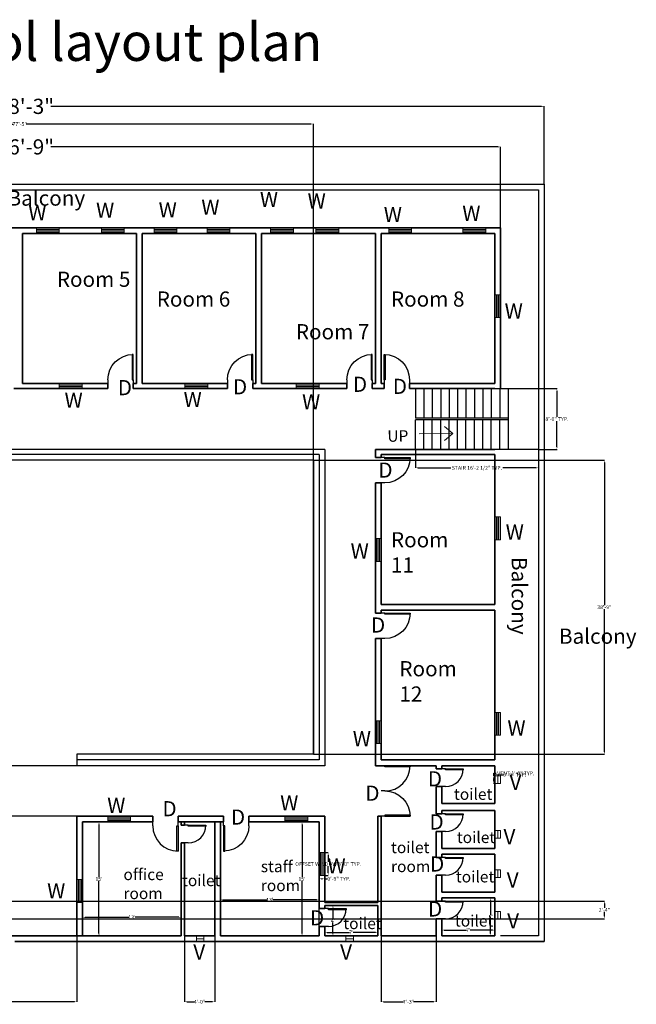
# Model space of a CAD drawing. Units: inches. Extents: x 6562 to 8578, y 2662 to 4218.
# Tile 3 of 3: x 7603 to 8578, y 2662 to 4218. Entities that reach past the tile are written whole.
import ezdxf

# ---------------------------------------------------------------- set-up
doc = ezdxf.new("R2010")
doc.units = ezdxf.units.IN
doc.header["$MEASUREMENT"] = 0
for name, color, linetype, lineweight in [('A-ANNO-DIMS', 2, 'Continuous', 18), ('A-ANNO-SYMB', 2, 'Continuous', 18), ('A-ANNO-TEXT', 7, 'Continuous', 18), ('A-AREA-IDEN', 7, 'Continuous', 25), ('A-DOOR', 3, 'Continuous', 25), ('A-FLOR-EDGE', 8, 'Continuous', 25), ('A-FLOR-STRS', 7, 'Continuous', 25), ('A-GLAZ', 4, 'Continuous', 18), ('A-GLAZ-VENT', 4, 'Continuous', 18), ('A-WALL', 7, 'Continuous', 35)]:
    doc.layers.add(name, color=color, linetype=linetype, lineweight=lineweight)
doc.styles.get("Standard").update_dxf_attribs({"font": 'arial.ttf'})
doc.dimstyles.get("Standard").update_dxf_attribs({"dimtxt": 6, "dimasz": 4, "dimexe": 0.18, "dimexo": 0.0625, "dimgap": 0.09, "dimtad": 0, "dimtih": 1, "dimtoh": 1, "dimdec": 0, "dimzin": 0, "dimdsep": 46, "dimlunit": 3, "dimtxsty": 'Standard', "dimcen": 0.09, "dimadec": 0, "dimazin": 0, "dimtfac": 1, "dimtdec": 0, "dimtofl": 0, "dimtmove": 0, "dimatfit": 3, "dimfxl": 1, "dimtolj": 1, "dimtzin": 0, "dimarcsym": 0})

# ---------------------------------------------------------------- blocks, each defined once
blk = doc.blocks.new('*U4')
for p, q in [((-40, 0), (-40, 6)), ((0, 0), (0, 6))]:
    blk.add_line(p, q)
blk.add_lwpolyline([(0, 0), (0, -40), (-1.75, -40), (-1.75, 0)], close=True)
blk.add_arc((0, 0), 40, 180, 270)
blk = doc.blocks.new('*U5')
for p, q in [((-28, 0), (-28, 6)), ((0, 0), (0, 6))]:
    blk.add_line(p, q)
blk.add_lwpolyline([(0, 0), (0, -28), (-1.75, -28), (-1.75, 0)], close=True)
blk.add_arc((0, 0), 28, 180, 270)
blk = doc.blocks.new('*U2')
for p, q in [((0, 0), (0, -6)), ((40, 0), (40, -6))]:
    blk.add_line(p, q)
blk.add_lwpolyline([(0, 0), (0, 40), (1.75, 40), (1.75, 0)], close=True)
blk.add_arc((0, 0), 40, 0, 90)
blk = doc.blocks.new('*U6')
for p, q in [((0, 0), (0, -6)), ((28, 0), (28, -6))]:
    blk.add_line(p, q)
blk.add_lwpolyline([(0, 0), (0, 28), (1.75, 28), (1.75, 0)], close=True)
blk.add_arc((0, 0), 28, 0, 90)
blk = doc.blocks.new('*U8')
for p, q in [((0, 0), (0, -6)), ((40, 0), (40, -6))]:
    blk.add_line(p, q)
blk.add_lwpolyline([(0, 0), (0, 40), (1.75, 40), (1.75, 0)], close=True)
blk.add_arc((0, 0), 40, 0, 90)
blk = doc.blocks.new('*U9')
for p, q in [((0, 0), (0, -6)), ((-40, 0), (-40, -6))]:
    blk.add_line(p, q)
blk.add_lwpolyline([(0, 0), (0, 40), (-1.75, 40), (-1.75, 0)], close=True)
blk.add_arc((0, 0), 40, 90, 180)
blk = doc.blocks.new('*U10')
for p, q in [((0, 0), (0, 6)), ((40, 0), (40, 6))]:
    blk.add_line(p, q)
blk.add_lwpolyline([(0, 0), (0, -40), (1.75, -40), (1.75, 0)], close=True)
blk.add_arc((0, 0), 40, 270, 0)
blk = doc.blocks.new('*D11')
at = {"layer": 'A-ANNO-DIMS', "color": 0, "lineweight": -2, "transparency": 16777216}
for p, q in [((6773.2, 3958.1), (6773.2, 4081.4)), ((6777.2, 4081.2), (7553.2, 4081.2)), ((8428.2, 4081.2), (7652.2, 4081.2)), ((8432.2, 3958.1), (8432.2, 4081.4))]:
    blk.add_line(p, q, dxfattribs=at)
at = {"layer": 'A-ANNO-DIMS', "color": 0, "transparency": 16777216}
for points in [[(6777.2, 4081.9), (6777.2, 4080.6), (6773.2, 4081.2)], [(8428.2, 4081.9), (8428.2, 4080.6), (8432.2, 4081.2)]]:
    blk.add_solid(points, dxfattribs=at)
at = {"layer": 'Defpoints', "color": 0, "transparency": 16777216}
for p in [(8432.2, 4081.2), (6773.2, 3958), (8432.2, 3958)]:
    blk.add_point(p, dxfattribs=at)
at = {"layer": 'A-ANNO-DIMS', "color": 0, "transparency": 16777216, "insert": (7602.7, 4081.2), "char_height": 6, "attachment_point": 5}
blk.add_mtext('\\A1;{\\H4x;138\'-3"}', dxfattribs=at)
blk = doc.blocks.new('*D12')
at = {"layer": 'A-ANNO-DIMS', "color": 0, "lineweight": -2, "transparency": 16777216}
for p, q in [((6842.2, 3889.1), (6842.2, 4017.3)), ((6846.2, 4017.1), (7553.2, 4017.1)), ((8359.2, 4017.1), (7652.2, 4017.1)), ((8363.2, 3889.1), (8363.2, 4017.3))]:
    blk.add_line(p, q, dxfattribs=at)
at = {"layer": 'A-ANNO-DIMS', "color": 0, "transparency": 16777216}
for points in [[(6846.2, 4017.8), (6846.2, 4016.4), (6842.2, 4017.1)], [(8359.2, 4017.8), (8359.2, 4016.4), (8363.2, 4017.1)]]:
    blk.add_solid(points, dxfattribs=at)
at = {"layer": 'Defpoints', "color": 0, "transparency": 16777216}
for p in [(8363.2, 4017.1), (6842.2, 3889), (8363.2, 3889)]:
    blk.add_point(p, dxfattribs=at)
at = {"layer": 'A-ANNO-DIMS', "color": 0, "transparency": 16777216, "insert": (7602.7, 4017.1), "char_height": 6, "attachment_point": 5}
blk.add_mtext('\\A1;{\\H4x;126\'-9"}', dxfattribs=at)
blk = doc.blocks.new('*D17')
at = {"layer": 'A-ANNO-DIMS', "color": 0, "lineweight": -2, "transparency": 16777216}
for p, q in [((7702.2, 2770.1), (7702.2, 2799.6)), ((7706.2, 2799.4), (7775.3, 2799.4)), ((7854.2, 2799.4), (7785.1, 2799.4)), ((7858.2, 2770.1), (7858.2, 2799.6))]:
    blk.add_line(p, q, dxfattribs=at)
at = {"layer": 'A-ANNO-DIMS', "color": 0, "transparency": 16777216}
for points in [[(7706.2, 2800.1), (7706.2, 2798.8), (7702.2, 2799.4)], [(7854.2, 2800.1), (7854.2, 2798.8), (7858.2, 2799.4)]]:
    blk.add_solid(points, dxfattribs=at)
at = {"layer": 'Defpoints', "color": 0, "transparency": 16777216}
for p in [(7858.2, 2799.4), (7702.2, 2770), (7858.2, 2770)]:
    blk.add_point(p, dxfattribs=at)
at = {"layer": 'A-ANNO-DIMS', "color": 0, "transparency": 16777216, "insert": (7780.2, 2799.4), "char_height": 6, "attachment_point": 5}
blk.add_mtext("\\A1;13'", dxfattribs=at)
blk = doc.blocks.new('*D18')
at = {"layer": 'A-ANNO-DIMS', "color": 0, "lineweight": -2, "transparency": 16777216}
for p, q in [((7702.2, 2950), (7728.3, 2950)), ((7728.1, 2946), (7728.1, 2863.2)), ((7728.1, 2774), (7728.1, 2856.8)), ((7702.2, 2770), (7728.3, 2770))]:
    blk.add_line(p, q, dxfattribs=at)
at = {"layer": 'A-ANNO-DIMS', "color": 0, "transparency": 16777216}
for points in [[(7727.5, 2946), (7728.8, 2946), (7728.1, 2950)], [(7727.5, 2774), (7728.8, 2774), (7728.1, 2770)]]:
    blk.add_solid(points, dxfattribs=at)
at = {"layer": 'Defpoints', "color": 0, "transparency": 16777216}
for p in [(7702.2, 2950), (7702.2, 2770), (7728.1, 2770)]:
    blk.add_point(p, dxfattribs=at)
at = {"layer": 'A-ANNO-DIMS', "color": 0, "transparency": 16777216, "insert": (7728.1, 2860), "char_height": 6, "attachment_point": 5}
blk.add_mtext("\\A1;15'", dxfattribs=at)
blk = doc.blocks.new('*D21')
at = {"layer": 'A-ANNO-DIMS', "color": 0, "lineweight": -2, "transparency": 16777216}
for p, q in [((7920.2, 2770.1), (7920.2, 2827.1)), ((7924.2, 2826.9), (7993.3, 2826.9)), ((8072.2, 2826.9), (8003.1, 2826.9)), ((8076.2, 2770.1), (8076.2, 2827.1))]:
    blk.add_line(p, q, dxfattribs=at)
at = {"layer": 'A-ANNO-DIMS', "color": 0, "transparency": 16777216}
for points in [[(7924.2, 2827.6), (7924.2, 2826.2), (7920.2, 2826.9)], [(8072.2, 2827.6), (8072.2, 2826.2), (8076.2, 2826.9)]]:
    blk.add_solid(points, dxfattribs=at)
at = {"layer": 'Defpoints', "color": 0, "transparency": 16777216}
for p in [(8076.2, 2826.9), (7920.2, 2770), (8076.2, 2770)]:
    blk.add_point(p, dxfattribs=at)
at = {"layer": 'A-ANNO-DIMS', "color": 0, "transparency": 16777216, "insert": (7998.2, 2826.9), "char_height": 6, "attachment_point": 5}
blk.add_mtext("\\A1;13'", dxfattribs=at)
blk = doc.blocks.new('*D22')
at = {"layer": 'A-ANNO-DIMS', "color": 0, "lineweight": -2, "transparency": 16777216}
for p, q in [((8076.1, 2950), (8049.1, 2950)), ((8049.2, 2946), (8049.2, 2863.2)), ((8049.2, 2774), (8049.2, 2856.8)), ((8076.1, 2770), (8049.1, 2770))]:
    blk.add_line(p, q, dxfattribs=at)
at = {"layer": 'A-ANNO-DIMS', "color": 0, "transparency": 16777216}
for points in [[(8048.6, 2946), (8049.9, 2946), (8049.2, 2950)], [(8048.6, 2774), (8049.9, 2774), (8049.2, 2770)]]:
    blk.add_solid(points, dxfattribs=at)
at = {"layer": 'Defpoints', "color": 0, "transparency": 16777216}
for p in [(8076.2, 2950), (8049.2, 2770), (8076.2, 2770)]:
    blk.add_point(p, dxfattribs=at)
at = {"layer": 'A-ANNO-DIMS', "color": 0, "transparency": 16777216, "insert": (8049.2, 2860), "char_height": 6, "attachment_point": 5}
blk.add_mtext("\\A1;15'", dxfattribs=at)
blk = doc.blocks.new('*D23')
at = {"layer": 'A-ANNO-DIMS', "color": 0, "lineweight": -2, "transparency": 16777216}
for p, q in [((8169.1, 2818), (8098, 2818)), ((8098.2, 2814), (8098.2, 2797.1)), ((8098.2, 2774), (8098.2, 2790.9)), ((8169.1, 2770), (8098, 2770))]:
    blk.add_line(p, q, dxfattribs=at)
at = {"layer": 'A-ANNO-DIMS', "color": 0, "transparency": 16777216}
for points in [[(8097.5, 2814), (8098.8, 2814), (8098.2, 2818)], [(8097.5, 2774), (8098.8, 2774), (8098.2, 2770)]]:
    blk.add_solid(points, dxfattribs=at)
at = {"layer": 'Defpoints', "color": 0, "transparency": 16777216}
for p in [(8169.2, 2818), (8098.2, 2770), (8169.2, 2770)]:
    blk.add_point(p, dxfattribs=at)
at = {"layer": 'A-ANNO-DIMS', "color": 0, "transparency": 16777216, "insert": (8098.2, 2794), "char_height": 6, "attachment_point": 5}
blk.add_mtext("\\A1;4'", dxfattribs=at)
blk = doc.blocks.new('*D24')
at = {"layer": 'A-ANNO-DIMS', "color": 0, "lineweight": -2, "transparency": 16777216}
for p, q in [((8085.2, 2770.1), (8085.2, 2775.7)), ((8089.2, 2775.5), (8124.4, 2775.5)), ((8165.2, 2775.5), (8130, 2775.5)), ((8169.2, 2770.1), (8169.2, 2775.7))]:
    blk.add_line(p, q, dxfattribs=at)
at = {"layer": 'A-ANNO-DIMS', "color": 0, "transparency": 16777216}
for points in [[(8089.2, 2776.1), (8089.2, 2774.8), (8085.2, 2775.5)], [(8165.2, 2776.1), (8165.2, 2774.8), (8169.2, 2775.5)]]:
    blk.add_solid(points, dxfattribs=at)
at = {"layer": 'Defpoints', "color": 0, "transparency": 16777216}
for p in [(8169.2, 2775.5), (8085.2, 2770), (8169.2, 2770)]:
    blk.add_point(p, dxfattribs=at)
at = {"layer": 'A-ANNO-DIMS', "color": 0, "transparency": 16777216, "insert": (8127.2, 2775.5), "char_height": 6, "attachment_point": 5}
blk.add_mtext("\\A1;7'", dxfattribs=at)
blk = doc.blocks.new('*D25')
at = {"layer": 'A-ANNO-DIMS', "color": 0, "lineweight": -2, "transparency": 16777216}
for p, q in [((8270.2, 2770.1), (8270.2, 2779.3)), ((8274.2, 2779.1), (8309.4, 2779.1)), ((8350.2, 2779.1), (8315, 2779.1)), ((8354.2, 2770.1), (8354.2, 2779.3))]:
    blk.add_line(p, q, dxfattribs=at)
at = {"layer": 'A-ANNO-DIMS', "color": 0, "transparency": 16777216}
for points in [[(8274.2, 2779.8), (8274.2, 2778.4), (8270.2, 2779.1)], [(8350.2, 2779.8), (8350.2, 2778.4), (8354.2, 2779.1)]]:
    blk.add_solid(points, dxfattribs=at)
at = {"layer": 'Defpoints', "color": 0, "transparency": 16777216}
for p in [(8354.2, 2779.1), (8270.2, 2770), (8354.2, 2770)]:
    blk.add_point(p, dxfattribs=at)
at = {"layer": 'A-ANNO-DIMS', "color": 0, "transparency": 16777216, "insert": (8312.2, 2779.1), "char_height": 6, "attachment_point": 5}
blk.add_mtext("\\A1;7'", dxfattribs=at)
blk = doc.blocks.new('*D26')
at = {"layer": 'A-ANNO-DIMS', "color": 0, "lineweight": -2, "transparency": 16777216}
for p, q in [((8354.1, 2830), (8347.2, 2830)), ((8347.4, 2826), (8347.4, 2803.1)), ((8347.4, 2774), (8347.4, 2796.9)), ((8354.1, 2770), (8347.2, 2770))]:
    blk.add_line(p, q, dxfattribs=at)
at = {"layer": 'A-ANNO-DIMS', "color": 0, "transparency": 16777216}
for points in [[(8346.7, 2826), (8348, 2826), (8347.4, 2830)], [(8346.7, 2774), (8348, 2774), (8347.4, 2770)]]:
    blk.add_solid(points, dxfattribs=at)
at = {"layer": 'Defpoints', "color": 0, "transparency": 16777216}
for p in [(8354.2, 2830), (8347.4, 2770), (8354.2, 2770)]:
    blk.add_point(p, dxfattribs=at)
at = {"layer": 'A-ANNO-DIMS', "color": 0, "transparency": 16777216, "insert": (8347.4, 2800), "char_height": 6, "attachment_point": 5}
blk.add_mtext("\\A1;5'", dxfattribs=at)
blk = doc.blocks.new('WIN-36-FRAMED')
for p, q in [((2.5, 36), (2.5, 0)), ((4.5, 36), (4.5, 0)), ((6.5, 36), (6.5, 0))]:
    blk.add_line(p, q)
blk.add_lwpolyline([(0, 36), (9, 36), (9, 0), (0, 0)], close=True)
blk = doc.blocks.new('STAIR-HALF-TURN')
for p, q in [((0, 96), (194.7, 96)), ((0, 96), (0, 49.3)), ((13.3, 96), (13.3, 49.3)), ((26.7, 96), (26.7, 49.3)), ((40, 96), (40, 49.3)), ((53.3, 96), (53.3, 49.3)), ((66.7, 96), (66.7, 49.3)), ((80, 96), (80, 49.3)), ((93.3, 96), (93.3, 49.3)), ((106.7, 96), (106.7, 49.3)), ((120, 96), (120, 49.3)), ((133.3, 96), (133.3, 49.3)), ((146.7, 96), (146.7, 48)), ((194.7, 96), (194.7, 48)), ((146.7, 49.3), (0, 49.3)), ((146.7, 48), (146.7, 0)), ((194.7, 48), (194.7, 0)), ((0, 0), (0, 46.7)), ((146.7, 46.7), (0, 46.7)), ((13.3, 0), (13.3, 46.7)), ((26.7, 0), (26.7, 46.7)), ((40, 0), (40, 46.7)), ((53.3, 0), (53.3, 46.7)), ((66.7, 0), (66.7, 46.7)), ((80, 0), (80, 46.7)), ((93.3, 0), (93.3, 46.7)), ((106.7, 0), (106.7, 46.7)), ((120, 0), (120, 46.7)), ((133.3, 0), (133.3, 46.7)), ((194.7, 0), (0, 0))]:
    blk.add_line(p, q)
blk = doc.blocks.new('VENT-12')
blk.add_line((4.5, 12), (4.5, 0))
blk.add_lwpolyline([(0, 12), (9, 12), (9, 0), (0, 0)], close=True)
blk = doc.blocks.new('WIN-36-VERANDA')
for p, q in [((0, 0), (0, 7.9)), ((36, 5.5), (0, 5.5)), ((36, 3.5), (0, 3.5)), ((36, 1.5), (0, 1.5)), ((36, 8), (36, 0))]:
    blk.add_line(p, q)
blk = doc.blocks.new('ARROW-STAIR-UP')
for p, q in [((0, 11.1), (13.3, 22.2)), ((53.3, 11.1), (0, 11.1)), ((0, 11.1), (13.3, 0))]:
    blk.add_line(p, q)
blk = doc.blocks.new('WIN-36-OFFSET')
for p, q in [((2.5, 36), (2.5, 0)), ((4.5, 36), (4.5, 0)), ((6.5, 36), (6.5, 0))]:
    blk.add_line(p, q)
blk.add_lwpolyline([(0, 36), (9, 36), (9, 0), (0, 0)], close=True)
blk = doc.blocks.new('*D37')
at = {"layer": 'A-ANNO-DIMS', "color": 0, "lineweight": -2, "transparency": 16777216}
for p, q in [((8085.2, 2901.6), (8090.8, 2901.6)), ((8090.6, 2897.6), (8090.6, 2886.8)), ((8090.6, 2869.6), (8090.6, 2880.4)), ((8085.2, 2865.6), (8090.8, 2865.6))]:
    blk.add_line(p, q, dxfattribs=at)
at = {"layer": 'A-ANNO-DIMS', "color": 0, "transparency": 16777216}
for points in [[(8089.9, 2897.6), (8091.2, 2897.6), (8090.6, 2901.6)], [(8089.9, 2869.6), (8091.2, 2869.6), (8090.6, 2865.6)]]:
    blk.add_solid(points, dxfattribs=at)
at = {"layer": 'Defpoints', "color": 0, "transparency": 16777216}
for p in [(8085.2, 2901.6), (8090.6, 2901.6), (8085.2, 2865.6)]:
    blk.add_point(p, dxfattribs=at)
at = {"layer": 'A-ANNO-DIMS', "color": 0, "transparency": 16777216, "insert": (8090.6, 2883.6), "char_height": 6, "attachment_point": 5}
blk.add_mtext('\\A1;OFFSET WINDOW 3\'-0" TYP.', dxfattribs=at)
blk = doc.blocks.new('*D38')
at = {"layer": 'A-ANNO-DIMS', "color": 0, "lineweight": -2, "transparency": 16777216}
for p, q in [((8076.2, 2865.5), (8076.2, 2860)), ((8085.2, 2865.5), (8085.2, 2860)), ((8080.2, 2860.2), (8081.2, 2860.2)), ((8085.2, 2860.2), (8089.2, 2860.2))]:
    blk.add_line(p, q, dxfattribs=at)
at = {"layer": 'A-ANNO-DIMS', "color": 0, "transparency": 16777216}
for points in [[(8080.2, 2860.9), (8080.2, 2859.5), (8076.2, 2860.2)], [(8081.2, 2860.9), (8081.2, 2859.5), (8085.2, 2860.2)]]:
    blk.add_solid(points, dxfattribs=at)
at = {"layer": 'Defpoints', "color": 0, "transparency": 16777216}
for p in [(8076.2, 2865.6), (8085.2, 2865.6), (8085.2, 2860.2)]:
    blk.add_point(p, dxfattribs=at)
at = {"layer": 'A-ANNO-DIMS', "color": 0, "transparency": 16777216, "insert": (8107.6, 2860.2), "char_height": 6, "attachment_point": 5}
blk.add_mtext('\\A1;0\'-9" TYP.', dxfattribs=at)
blk = doc.blocks.new('*D41')
at = {"layer": 'A-ANNO-DIMS', "color": 0, "lineweight": -2, "transparency": 16777216}
for p, q in [((8354.1, 3023), (8352.2, 3023)), ((8352.4, 3023), (8352.4, 3027)), ((8352.4, 3027), (8356.4, 3027)), ((8354.1, 3011), (8352.2, 3011)), ((8352.4, 3015), (8352.4, 3019))]:
    blk.add_line(p, q, dxfattribs=at)
at = {"layer": 'A-ANNO-DIMS', "color": 0, "transparency": 16777216}
for points in [[(8351.7, 3019), (8353, 3019), (8352.4, 3023)], [(8351.7, 3015), (8353, 3015), (8352.4, 3011)]]:
    blk.add_solid(points, dxfattribs=at)
at = {"layer": 'Defpoints', "color": 0, "transparency": 16777216}
for p in [(8352.4, 3023), (8354.2, 3023), (8354.2, 3011)]:
    blk.add_point(p, dxfattribs=at)
at = {"layer": 'A-ANNO-DIMS', "color": 0, "transparency": 16777216, "insert": (8387.3, 3027), "char_height": 6, "attachment_point": 5}
blk.add_mtext('\\A1;VENT 1\'-0" TYP.', dxfattribs=at)
blk = doc.blocks.new('*D42')
at = {"layer": 'A-ANNO-DIMS', "color": 0, "lineweight": -2, "transparency": 16777216}
for p, q in [((8354.2, 3023), (8354.2, 3025)), ((8358.2, 3024.8), (8359.2, 3024.8)), ((8363.2, 3023), (8363.2, 3025)), ((8363.2, 3024.8), (8367.2, 3024.8))]:
    blk.add_line(p, q, dxfattribs=at)
at = {"layer": 'A-ANNO-DIMS', "color": 0, "transparency": 16777216}
for points in [[(8358.2, 3025.5), (8358.2, 3024.1), (8354.2, 3024.8)], [(8359.2, 3025.5), (8359.2, 3024.1), (8363.2, 3024.8)]]:
    blk.add_solid(points, dxfattribs=at)
at = {"layer": 'Defpoints', "color": 0, "transparency": 16777216}
for p in [(8354.2, 3023), (8363.2, 3024.8), (8363.2, 3023)]:
    blk.add_point(p, dxfattribs=at)
at = {"layer": 'A-ANNO-DIMS', "color": 0, "transparency": 16777216, "insert": (8385.6, 3024.8), "char_height": 6, "attachment_point": 5}
blk.add_mtext('\\A1;0\'-9" TYP.', dxfattribs=at)
blk = doc.blocks.new('*D43')
at = {"layer": 'A-ANNO-DIMS', "color": 0, "lineweight": -2, "transparency": 16777216}
for p, q in [((8228.5, 3538.9), (8228.5, 3509.6)), ((8423.2, 3538.9), (8423.2, 3509.6)), ((8232.5, 3509.8), (8284.7, 3509.8)), ((8419.2, 3509.8), (8367, 3509.8))]:
    blk.add_line(p, q, dxfattribs=at)
at = {"layer": 'A-ANNO-DIMS', "color": 0, "transparency": 16777216}
for points in [[(8232.5, 3510.5), (8232.5, 3509.1), (8228.5, 3509.8)], [(8419.2, 3510.5), (8419.2, 3509.1), (8423.2, 3509.8)]]:
    blk.add_solid(points, dxfattribs=at)
at = {"layer": 'Defpoints', "color": 0, "transparency": 16777216}
for p in [(8228.5, 3539), (8423.2, 3539), (8423.2, 3509.8)]:
    blk.add_point(p, dxfattribs=at)
at = {"layer": 'A-ANNO-DIMS', "color": 0, "transparency": 16777216, "insert": (8325.8, 3509.8), "char_height": 6, "attachment_point": 5}
blk.add_mtext('\\A1;STAIR 16\'-2 1/2" TYP.', dxfattribs=at)
blk = doc.blocks.new('*D44')
at = {"layer": 'A-ANNO-DIMS', "color": 0, "lineweight": -2, "transparency": 16777216}
for p, q in [((8423.2, 3635), (8452.6, 3635)), ((8452.4, 3631), (8452.4, 3590.2)), ((8452.4, 3543), (8452.4, 3583.8)), ((8423.2, 3539), (8452.6, 3539))]:
    blk.add_line(p, q, dxfattribs=at)
at = {"layer": 'A-ANNO-DIMS', "color": 0, "transparency": 16777216}
for points in [[(8451.7, 3631), (8453, 3631), (8452.4, 3635)], [(8451.7, 3543), (8453, 3543), (8452.4, 3539)]]:
    blk.add_solid(points, dxfattribs=at)
at = {"layer": 'Defpoints', "color": 0, "transparency": 16777216}
for p in [(8423.2, 3635), (8452.4, 3635), (8423.2, 3539)]:
    blk.add_point(p, dxfattribs=at)
at = {"layer": 'A-ANNO-DIMS', "color": 0, "transparency": 16777216, "insert": (8452.4, 3587), "char_height": 6, "attachment_point": 5}
blk.add_mtext('\\A1;8\'-0" TYP.', dxfattribs=at)
blk = doc.blocks.new('*D45')
at = {"layer": 'A-ANNO-DIMS', "color": 0, "lineweight": -2, "transparency": 16777216}
for p, q in [((7138.2, 2935.1), (7138.2, 4053.4)), ((7142.2, 4053.3), (7592.3, 4053.3)), ((8063.2, 4053.3), (7613, 4053.3)), ((8067.2, 3057.1), (8067.2, 4053.4))]:
    blk.add_line(p, q, dxfattribs=at)
at = {"layer": 'A-ANNO-DIMS', "color": 0, "transparency": 16777216}
for points in [[(7142.2, 4053.9), (7142.2, 4052.6), (7138.2, 4053.3)], [(8063.2, 4053.9), (8063.2, 4052.6), (8067.2, 4053.3)]]:
    blk.add_solid(points, dxfattribs=at)
at = {"layer": 'Defpoints', "color": 0, "transparency": 16777216}
for p in [(8067.2, 4053.3), (8067.2, 3057), (7138.2, 2935)]:
    blk.add_point(p, dxfattribs=at)
at = {"layer": 'A-ANNO-DIMS', "color": 0, "transparency": 16777216, "insert": (7602.7, 4053.3), "char_height": 6, "attachment_point": 5}
blk.add_mtext('\\A1;77\'-5"', dxfattribs=at)
blk = doc.blocks.new('*D46')
at = {"layer": 'A-ANNO-DIMS', "color": 0, "lineweight": -2, "transparency": 16777216}
for p, q in [((8067.2, 3522), (8527.6, 3522)), ((8527.4, 3518), (8527.4, 3292.7)), ((8527.4, 3061), (8527.4, 3286.3)), ((8067.2, 3057), (8527.6, 3057))]:
    blk.add_line(p, q, dxfattribs=at)
at = {"layer": 'A-ANNO-DIMS', "color": 0, "transparency": 16777216}
for points in [[(8526.8, 3518), (8528.1, 3518), (8527.4, 3522)], [(8526.8, 3061), (8528.1, 3061), (8527.4, 3057)]]:
    blk.add_solid(points, dxfattribs=at)
at = {"layer": 'Defpoints', "color": 0, "transparency": 16777216}
for p in [(8067.2, 3522), (8527.4, 3522), (8067.2, 3057)]:
    blk.add_point(p, dxfattribs=at)
at = {"layer": 'A-ANNO-DIMS', "color": 0, "transparency": 16777216, "insert": (8527.4, 3289.5), "char_height": 6, "attachment_point": 5}
blk.add_mtext('\\A1;38\'-9"', dxfattribs=at)
blk = doc.blocks.new('*D49')
at = {"layer": 'A-ANNO-DIMS', "color": 0, "lineweight": -2, "transparency": 16777216}
for p, q in [((7353.2, 2769.9), (7353.2, 2665.6)), ((7693.2, 2769.9), (7693.2, 2665.6)), ((7357.2, 2665.8), (7512.7, 2665.8)), ((7689.2, 2665.8), (7533.6, 2665.8))]:
    blk.add_line(p, q, dxfattribs=at)
at = {"layer": 'A-ANNO-DIMS', "color": 0, "transparency": 16777216}
for points in [[(7357.2, 2666.4), (7357.2, 2665.1), (7353.2, 2665.8)], [(7689.2, 2666.4), (7689.2, 2665.1), (7693.2, 2665.8)]]:
    blk.add_solid(points, dxfattribs=at)
at = {"layer": 'Defpoints', "color": 0, "transparency": 16777216}
for p in [(7353.2, 2770), (7693.2, 2770), (7693.2, 2665.8)]:
    blk.add_point(p, dxfattribs=at)
at = {"layer": 'A-ANNO-DIMS', "color": 0, "transparency": 16777216, "insert": (7523.2, 2665.8), "char_height": 6, "attachment_point": 5}
blk.add_mtext('\\A1;28\'-4"', dxfattribs=at)
blk = doc.blocks.new('*D51')
at = {"layer": 'A-ANNO-DIMS', "color": 0, "lineweight": -2, "transparency": 16777216}
for p, q in [((6935.2, 2825), (8527.6, 2825)), ((8527.4, 2821), (8527.4, 2814.1)), ((8527.4, 2801), (8527.4, 2807.9)), ((6935.2, 2797), (8527.6, 2797))]:
    blk.add_line(p, q, dxfattribs=at)
at = {"layer": 'A-ANNO-DIMS', "color": 0, "transparency": 16777216}
for points in [[(8526.8, 2821), (8528.1, 2821), (8527.4, 2825)], [(8526.8, 2801), (8528.1, 2801), (8527.4, 2797)]]:
    blk.add_solid(points, dxfattribs=at)
at = {"layer": 'Defpoints', "color": 0, "transparency": 16777216}
for p in [(6935.2, 2825), (8527.4, 2825), (6935.2, 2797)]:
    blk.add_point(p, dxfattribs=at)
at = {"layer": 'A-ANNO-DIMS', "color": 0, "transparency": 16777216, "insert": (8527.4, 2811), "char_height": 6, "attachment_point": 5}
blk.add_mtext('\\A1;2\'-4"', dxfattribs=at)
blk = doc.blocks.new('*D55')
at = {"layer": 'A-ANNO-DIMS', "color": 0, "lineweight": -2, "transparency": 16777216}
for p, q in [((7863.2, 2769.9), (7863.2, 2665.6)), ((7911.2, 2769.9), (7911.2, 2665.6)), ((7867.2, 2665.8), (7879, 2665.8)), ((7907.2, 2665.8), (7895.4, 2665.8))]:
    blk.add_line(p, q, dxfattribs=at)
at = {"layer": 'A-ANNO-DIMS', "color": 0, "transparency": 16777216}
for points in [[(7867.2, 2666.4), (7867.2, 2665.1), (7863.2, 2665.8)], [(7907.2, 2666.4), (7907.2, 2665.1), (7911.2, 2665.8)]]:
    blk.add_solid(points, dxfattribs=at)
at = {"layer": 'Defpoints', "color": 0, "transparency": 16777216}
for p in [(7863.2, 2770), (7911.2, 2770), (7911.2, 2665.8)]:
    blk.add_point(p, dxfattribs=at)
at = {"layer": 'A-ANNO-DIMS', "color": 0, "transparency": 16777216, "insert": (7887.2, 2665.8), "char_height": 6, "attachment_point": 5}
blk.add_mtext('\\A1;4\'-0"', dxfattribs=at)
blk = doc.blocks.new('*D56')
at = {"layer": 'A-ANNO-DIMS', "color": 0, "lineweight": -2, "transparency": 16777216}
for p, q in [((8174.2, 2769.9), (8174.2, 2665.6)), ((8261.2, 2769.9), (8261.2, 2665.6)), ((8178.2, 2665.8), (8209.6, 2665.8)), ((8257.2, 2665.8), (8225.7, 2665.8))]:
    blk.add_line(p, q, dxfattribs=at)
at = {"layer": 'A-ANNO-DIMS', "color": 0, "transparency": 16777216}
for points in [[(8178.2, 2666.4), (8178.2, 2665.1), (8174.2, 2665.8)], [(8257.2, 2666.4), (8257.2, 2665.1), (8261.2, 2665.8)]]:
    blk.add_solid(points, dxfattribs=at)
at = {"layer": 'Defpoints', "color": 0, "transparency": 16777216}
for p in [(8174.2, 2770), (8261.2, 2770), (8261.2, 2665.8)]:
    blk.add_point(p, dxfattribs=at)
at = {"layer": 'A-ANNO-DIMS', "color": 0, "transparency": 16777216, "insert": (8217.7, 2665.8), "char_height": 6, "attachment_point": 5}
blk.add_mtext('\\A1;7\'-3"', dxfattribs=at)
blk = doc.blocks.new('*D58')
at = {"layer": 'A-ANNO-DIMS', "color": 0, "lineweight": -2, "transparency": 16777216}
for p, q in [((7693.1, 3039), (6677.7, 3039)), ((6677.9, 3035), (6677.9, 3002.2)), ((6677.9, 2963), (6677.9, 2995.8)), ((7693.1, 2959), (6677.7, 2959))]:
    blk.add_line(p, q, dxfattribs=at)
at = {"layer": 'A-ANNO-DIMS', "color": 0, "transparency": 16777216}
for points in [[(6677.3, 3035), (6678.6, 3035), (6677.9, 3039)], [(6677.3, 2963), (6678.6, 2963), (6677.9, 2959)]]:
    blk.add_solid(points, dxfattribs=at)
at = {"layer": 'Defpoints', "color": 0, "transparency": 16777216}
for p in [(6677.9, 3039), (7693.2, 3039), (7693.2, 2959)]:
    blk.add_point(p, dxfattribs=at)
at = {"layer": 'A-ANNO-DIMS', "color": 0, "transparency": 16777216, "insert": (6677.9, 2999), "char_height": 6, "attachment_point": 5}
blk.add_mtext('\\A1;6\'-8"', dxfattribs=at)

msp = doc.modelspace()

# ---------------------------------------------------------------- linework, layer by layer
at = {"layer": 'A-FLOR-EDGE'}
for p, q in [((6773.18, 3958), (8432.18, 3958)), ((8432.18, 3958), (8432.18, 2761)), ((6782.18, 3949), (8423.18, 3949)), ((8423.18, 3949), (8423.18, 2770)), ((8085.18, 3539), (7120.18, 3539)), ((8085.18, 3539), (8085.18, 3039)), ((8076.18, 3531), (7129.17, 3531)), ((8067.18, 3522), (7138.17, 3522)), ((8067.18, 3522), (8067.18, 3057)), ((8076.18, 3531), (8076.18, 3048)), ((7693.18, 3057), (7693.18, 3039)), ((8067.18, 3057), (7693.18, 3057)), ((8076.18, 3048), (7693.18, 3048)), ((8085.18, 3039), (7693.18, 3039)), ((8423.18, 2770), (8363.18, 2770))]:
    msp.add_line(p, q, dxfattribs=at)
at = {"layer": 'A-WALL'}
for p, q in [((6842.18, 3889), (8363.18, 3889)), ((7607.18, 3880), (7607.18, 3643)), ((7607.18, 3880), (7787.18, 3880)), ((7787.18, 3880), (7787.18, 3643)), ((7796.18, 3880), (7796.18, 3643)), ((7796.18, 3880), (7976.18, 3880)), ((7976.18, 3880), (7976.18, 3643)), ((7985.18, 3880), (7985.18, 3643)), ((7985.18, 3880), (8165.18, 3880)), ((8165.18, 3880), (8165.18, 3643)), ((8165.18, 3880), (8165.18, 3643)), ((8174.18, 3880), (8174.18, 3643)), ((8174.18, 3880), (8354.18, 3880)), ((8354.18, 3880), (8354.18, 3643)), ((8363.18, 3889), (8363.18, 3635)), ((7742.18, 3643), (7607.18, 3643)), ((7742.18, 3643), (7742.18, 3643)), ((7742.18, 3643), (7742.18, 3635)), ((7787.18, 3643), (7782.18, 3643)), ((7782.18, 3643), (7782.18, 3635)), ((7931.18, 3643), (7796.18, 3643)), ((7931.18, 3643), (7931.18, 3635)), ((7976.18, 3643), (7971.18, 3643)), ((7971.18, 3643), (7971.18, 3635)), ((8120.18, 3643), (7985.18, 3643)), ((8120.18, 3643), (8120.18, 3635)), ((8165.18, 3643), (8160.18, 3643)), ((8160.18, 3643), (8160.18, 3635)), ((8179.18, 3643), (8174.18, 3643)), ((8179.18, 3643), (8179.18, 3635)), ((8354.18, 3643), (8219.18, 3643)), ((8219.18, 3643), (8219.18, 3635)), ((7742.18, 3635), (7593.18, 3635)), ((7931.18, 3635), (7782.18, 3635)), ((7931.18, 3635), (7931.18, 3635)), ((8120.18, 3635), (7971.18, 3635)), ((8179.18, 3635), (8160.18, 3635)), ((8354.18, 3635), (8219.18, 3635)), ((8354.18, 3539), (8165.18, 3539)), ((8165.18, 3539), (8165.18, 3526)), ((8174.18, 3526), (8165.18, 3526)), ((8354.18, 3531), (8174.18, 3531)), ((8174.18, 3531), (8174.18, 3526)), ((8354.18, 3531), (8354.18, 3294)), ((8174.18, 3486), (8165.18, 3486)), ((8165.18, 3486), (8165.18, 3486)), ((8165.18, 3486), (8165.18, 3280)), ((8174.18, 3486), (8174.18, 3294)), ((8165.18, 3285), (8165.18, 3280)), ((8354.18, 3294), (8174.18, 3294)), ((8354.18, 3285), (8174.18, 3285)), ((8174.18, 3285), (8174.18, 3280)), ((8354.18, 3285), (8354.18, 3048)), ((8174.18, 3280), (8165.18, 3280)), ((8174.18, 3240), (8165.18, 3240)), ((8165.18, 3240), (8165.18, 3039)), ((8165.18, 3240), (8165.18, 3048)), ((8174.18, 3240), (8174.18, 3048)), ((8261.18, 3039), (8165.18, 3039)), ((8220.18, 3039), (8169.18, 3039)), ((8354.18, 3048), (8174.18, 3048)), ((8261.18, 3039), (8261.18, 3034)), ((8270.18, 3039), (8270.18, 3034)), ((8354.18, 3039), (8270.18, 3039)), ((8354.18, 3039), (8354.18, 2979)), ((8270.18, 3034), (8261.18, 3034)), ((8270.18, 3006), (8261.18, 3006)), ((8261.18, 3006), (8261.18, 2963)), ((8270.18, 3006), (8270.18, 2979)), ((8354.18, 2979), (8270.18, 2979)), ((7813.18, 2959), (7693.18, 2959)), ((7813.18, 2959), (7693.18, 2959)), ((7693.18, 2959), (7693.18, 2770)), ((7813.18, 2950), (7813.18, 2959)), ((7853.18, 2950), (7853.18, 2959)), ((7925.18, 2959), (7853.18, 2959)), ((7925.18, 2959), (7853.18, 2959)), ((7925.18, 2950), (7925.18, 2959)), ((7965.18, 2950), (7965.18, 2959)), ((8076.18, 2959), (7965.18, 2959)), ((8076.18, 2959), (8085.18, 2959)), ((8085.18, 2959), (8085.18, 2823)), ((8174.18, 2959), (8169.18, 2959)), ((8169.18, 2959), (8174.18, 2959)), ((8169.18, 2959), (8169.18, 2823)), ((8174.18, 2959), (8174.18, 2770)), ((8220.18, 2960), (8220.16, 2960)), ((8270.18, 2963), (8261.18, 2963)), ((8270.18, 2968), (8270.18, 2963)), ((8354.18, 2968), (8270.18, 2968)), ((8354.18, 2968), (8354.18, 2908)), ((7813.18, 2950), (7702.18, 2950)), ((7702.18, 2950), (7702.18, 2770)), ((7858.18, 2950), (7853.18, 2950)), ((7858.18, 2950), (7858.18, 2945)), ((7925.18, 2950), (7858.18, 2950)), ((7863.18, 2945), (7858.18, 2945)), ((7863.18, 2950), (7863.18, 2945)), ((7911.18, 2950), (7863.18, 2950)), ((7875.18, 2950), (7870.18, 2950)), ((7911.18, 2950), (7911.18, 2770)), ((7920.18, 2950), (7920.18, 2770)), ((7925.18, 2950), (7920.18, 2950)), ((8076.18, 2950), (7965.18, 2950)), ((8076.18, 2950), (8076.18, 2813)), ((8270.18, 2935), (8261.18, 2935)), ((8261.18, 2935), (8261.18, 2894)), ((8270.18, 2935), (8270.18, 2908)), ((7863.18, 2917), (7858.18, 2917)), ((7858.18, 2917), (7858.18, 2770)), ((7863.18, 2917), (7863.18, 2770)), ((8354.18, 2908), (8270.18, 2908)), ((8354.18, 2899), (8270.18, 2899)), ((8270.18, 2899), (8270.18, 2894)), ((8354.18, 2899), (8354.18, 2839)), ((8270.18, 2894), (8261.18, 2894)), ((8270.18, 2866), (8261.18, 2866)), ((8261.18, 2866), (8261.18, 2825)), ((8270.18, 2866), (8270.18, 2839)), ((8354.18, 2839), (8270.18, 2839)), ((8169.18, 2823), (8085.18, 2823)), ((8085.18, 2818), (8085.18, 2813)), ((8169.18, 2818), (8085.18, 2818)), ((8169.18, 2818), (8169.18, 2770)), ((8270.18, 2825), (8261.18, 2825)), ((8354.18, 2830), (8270.18, 2830)), ((8270.18, 2830), (8270.18, 2825)), ((8354.18, 2830), (8354.18, 2770)), ((8085.18, 2813), (8076.18, 2813)), ((8270.18, 2797), (8261.18, 2797)), ((8261.18, 2797), (8261.18, 2770)), ((8270.18, 2797), (8270.18, 2770)), ((8085.18, 2785), (8076.18, 2785)), ((8076.18, 2785), (8076.18, 2770)), ((8085.18, 2785), (8085.18, 2770)), ((7353.17, 2770), (7693.18, 2770)), ((8432.18, 2761), (7595.18, 2761)), ((7705.18, 2770), (7670.18, 2770)), ((7858.18, 2770), (7702.18, 2770)), ((7911.18, 2770), (7863.18, 2770)), ((8076.18, 2770), (7920.18, 2770)), ((8169.18, 2770), (8085.18, 2770)), ((8261.18, 2770), (8174.18, 2770)), ((8354.18, 2770), (8270.18, 2770))]:
    msp.add_line(p, q, dxfattribs=at)

# ---------------------------------------------------------------- block references
at = {"layer": 'A-ANNO-SYMB', "rotation": 180.7954630467649}
msp.add_blockref('ARROW-STAIR-UP', (8287.74, 3575.36), dxfattribs=at)
at = {"layer": 'A-DOOR', "xscale": -1}
for name, p in [('*U8', (7782.18, 3649)), ('*U8', (7782.18, 3649)), ('*U8', (7971.18, 3649)), ('*U8', (8160.18, 3649)), ('*U9', (8179.18, 3649)), ('*U4', (7925.18, 2944))]:
    msp.add_blockref(name, p, dxfattribs=at)
for name, p, rotation in [('*U10', (8180.18, 3526), 90.00000000000384), ('*U10', (8180.18, 3280), 90.00000000000384), ('*U2', (8180.18, 2959), 270)]:
    msp.add_blockref(name, p, dxfattribs=dict(at, rotation=rotation))
at = {"layer": 'A-DOOR'}
for name, p, rotation in [('*U2', (8180.18, 3039), 270), ('*U6', (8276.18, 3034), 270), ('*U6', (8276.18, 2963), 270), ('*U5', (7869.18, 2945), 90), ('*U6', (8276.18, 2894), 270), ('*U6', (8276.18, 2825), 270), ('*U5', (8091.18, 2813), 90)]:
    msp.add_blockref(name, p, dxfattribs=dict(at, rotation=rotation))
msp.add_blockref('*U4', (7853.18, 2944), dxfattribs=at)
at = {"layer": 'A-FLOR-STRS'}
msp.add_blockref('STAIR-HALF-TURN', (8228.51, 3539), dxfattribs=at)
at = {"layer": 'A-GLAZ'}
for p, rotation in [((7629.24, 3889), 270.0000000000003), ((7731.93, 3889), 270.0000000000015), ((7815.18, 3889), 270.0000000000021), ((7899.28, 3889), 270.0000000000009), ((7999.47, 3889), 270.0000000000009), ((7999.47, 3889), 270.0000000000009), ((8071.28, 3889), 270.0000000000009), ((8186.45, 3889), 270.0000000000009), ((8303.67, 3889), 270.0000000000009), ((7741.97, 2959), 269.9999999999984), ((8022.14, 2959), 269.9999999999984)]:
    msp.add_blockref('WIN-36-FRAMED', p, dxfattribs=dict(at, rotation=rotation))
for name, p in [('WIN-36-FRAMED', (8354.18, 3747.24)), ('WIN-36-VERANDA', (7665.35, 3635)), ('WIN-36-VERANDA', (7864.01, 3635)), ('WIN-36-VERANDA', (8040.14, 3635)), ('WIN-36-VERANDA', (8040.14, 3635)), ('WIN-36-FRAMED', (8354.18, 3396.2)), ('WIN-36-FRAMED', (8165.18, 3361.87)), ('WIN-36-FRAMED', (8354.18, 3087.31)), ('WIN-36-FRAMED', (8165.18, 3073.91)), ('WIN-36-OFFSET', (8076.18, 2865.6)), ('WIN-36-OFFSET', (7693.18, 2822.89))]:
    msp.add_blockref(name, p, dxfattribs=at)
at = {"layer": 'A-GLAZ-VENT'}
for p in [(8354.18, 3010.99), (8354.18, 3010.99), (8354.18, 2924.52), (8354.18, 2924.52), (8354.18, 2862.51), (8354.18, 2862.51), (8354.18, 2796.3), (8354.18, 2796.3)]:
    msp.add_blockref('VENT-12', p, dxfattribs=at)
at = {"layer": 'A-GLAZ-VENT', "rotation": 269.9999999999976}
for p in [(7882.17, 2770), (8118.52, 2770)]:
    msp.add_blockref('VENT-12', p, dxfattribs=at)

# ---------------------------------------------------------------- texts
at = {"layer": 'A-ANNO-TEXT', "attachment_point": 1}
for s, width, insert, char_height in [('school layout plan', 1424.8444, (7380.26, 4213.03), 60), ('W', 32.1856, (7982.57, 3946.08), 24), ('W', 32.1856, (8058.02, 3943.63), 24), ('W', 32.1856, (7616.27, 3925.12), 24), ('W', 32.1856, (7723.49, 3929.01), 24), ('W', 32.1856, (7822.44, 3929.54), 24), ('W', 32.1856, (7889.93, 3933.83), 24), ('W', 32.1856, (8178.49, 3922.23), 24), ('W', 32.1856, (8302.66, 3924.2), 24), ('W', 32.1856, (8369.67, 3769.67), 24), ('D', 32.1856, (7757.82, 3648.61), 24), ('D', 32.1856, (7939.93, 3649.9), 24), ('D', 32.1856, (8129.64, 3653.93), 24), ('D', 32.1856, (8192.74, 3650.59), 24), ('W', 32.1856, (7673.64, 3628.73), 24), ('W', 32.1856, (7861.9, 3629.91), 24), ('W', 32.1856, (8049.3, 3626.24), 24), ('D', 32.1856, (8169.96, 3518.22), 24), ('W', 32.1856, (8371.31, 3420.33), 24), ('W', 32.1856, (8126.04, 3390.28), 24), ('D', 32.1856, (8158.32, 3273.38), 24), ('W', 32.1856, (8374.05, 3110.67), 24), ('W', 32.1856, (8129.49, 3093.71), 24), ('D', 32.1856, (8248.19, 3030.25), 24), ('V', 32.1856, (8377.44, 3024.72), 24), ('D', 32.1856, (8149.33, 3007.53), 24), ('W', 32.1856, (7741.12, 2988.45), 24), ('W', 32.1856, (8014.65, 2992.29), 24), ('D', 32.1856, (7828.42, 2982.93), 24), ('D', 32.1856, (7936.74, 2969.74), 24), ('D', 32.1856, (7936.74, 2969.74), 24), ('D', 32.1856, (8250.81, 2962.09), 24), ('V', 32.1856, (8367.83, 2938.91), 24), ('V', 32.1856, (8367.83, 2938.91), 24), ('D', 32.1856, (8251.68, 2895.68), 24), ('W', 32.1856, (8089.51, 2892.59), 24), ('V', 32.1856, (8372.95, 2870.38), 24), ('W', 32.1856, (7646.11, 2853.29), 24), ('D', 32.1856, (8248.49, 2824.6), 24), ('D', 32.1856, (8061.79, 2810.53), 24), ('V', 32.1856, (8373.6, 2805.7), 24), ('V', 32.1856, (7877.3, 2756.51), 24), ('V', 32.1856, (8109.44, 2756.39), 24)]:
    msp.add_mtext_dynamic_manual_height_columns(s, width=width, gutter_width=40, heights=[0], dxfattribs=dict(at, insert=insert, char_height=char_height))
at = {"layer": 'A-ANNO-TEXT', "insert": (8184.01, 3568.93), "char_height": 18, "attachment_point": 1, "rotation": 0.79546}
msp.add_mtext_dynamic_manual_height_columns('UP', width=38.7631, gutter_width=40, heights=[0], dxfattribs=at)
at = {"layer": 'A-AREA-IDEN', "attachment_point": 1}
for s, width, gutter_width, insert, char_height in [('Balcony', 33.181, 40, (7583.46, 3948.18), 24), ('Room 5', 125.7129, 1, (7661.46, 3819.9), 24), ('Room 6', 125.7129, 1, (7819.45, 3788.61), 24), ('Room 8', 125.7129, 1, (8189.88, 3788.61), 24), ('Room 7', 125.7129, 1, (8039.46, 3736.94), 24), ('Room 11', 125.7129, 1, (8189.88, 3408.1), 24), ('Balcony', 33.181, 40, (8455.52, 3255.71), 24), ('Room 12', 125.7129, 1, (8203.18, 3204.29), 24), ('toilet', 20.0644, 40, (8289.51, 3003), 18), ('toilet', 20.0644, 40, (8294.07, 2934.71), 18), ('toilet room', 20.0644, 40, (8189.99, 2918.77), 18), ('staff room', 20.0644, 40, (7984.03, 2888.67), 18), ('office room', 20.0644, 40, (7766.78, 2876.12), 18), ('toilet', 20.0644, 40, (7859.43, 2866.58), 18), ('toilet', 20.0644, 40, (7859.43, 2866.58), 18), ('toilet', 20.0644, 40, (8292.55, 2872.48), 18), ('toilet', 20.0644, 40, (8291.03, 2802.67), 18), ('toilet', 20.0644, 40, (8114.49, 2798.65), 18), ('toilet', 20.0644, 40, (8114.49, 2798.65), 18)]:
    msp.add_mtext_dynamic_manual_height_columns(s, width=width, gutter_width=gutter_width, heights=[0], dxfattribs=dict(at, insert=insert, char_height=char_height))
at = {"layer": 'A-AREA-IDEN', "insert": (8404.88, 3368.94), "char_height": 24, "attachment_point": 1, "rotation": 270}
msp.add_mtext_dynamic_manual_height_columns('Balcony', width=33.181, gutter_width=40, heights=[0], dxfattribs=at)
msp.add_mtext_dynamic_manual_height_columns('Balcony', width=33.181, gutter_width=40, heights=[0], dxfattribs=at)

# ---------------------------------------------------------------- dimensions: what is measured, and where the dimension line sits
at = {"layer": 'A-ANNO-DIMS'}
for base, p1, p2, text, override, picture, middle in [((8432.18, 4081.22), (6773.18, 3958), (8432.18, 3958), '{\\H4x;<>}', {"dimclrd": 0, "dimclre": 0, "dimclrt": 0}, '*D11', (7602.68, 4081.22)), ((8363.18, 4017.09), (6842.18, 3889), (8363.18, 3889), '{\\H4x;<>}', {"dimclrd": 0, "dimclre": 0, "dimclrt": 0}, '*D12', (7602.68, 4017.09)), ((8423.18, 3509.8), (8228.51, 3539), (8423.18, 3539), 'STAIR <> TYP.', {"dimdec": 1, "dimlfac": 1, "dimrnd": 0, "dimzin": 1, "dimdsep": 46, "dimlunit": 4, "dimfrac": 2}, '*D43', (8325.84, 3509.8)), ((8363.18, 3024.79), (8354.18, 3022.99), (8363.18, 3022.99), '<> TYP.', {"dimdec": 1, "dimlfac": 1, "dimrnd": 0, "dimzin": 1, "dimdsep": 46, "dimlunit": 4, "dimfrac": 2}, '*D42', (8385.55, 3024.79)), ((8085.18, 2860.2), (8076.18, 2865.6), (8085.18, 2865.6), '<> TYP.', {"dimdec": 1, "dimlfac": 1, "dimrnd": 0, "dimzin": 1, "dimdsep": 46, "dimlunit": 4, "dimfrac": 2}, '*D38', (8107.55, 2860.2))]:
    dim = msp.add_linear_dim(base=base, p1=p1, p2=p2, text=text, dimstyle='Standard', override=override, dxfattribs=at)
    dim.commit()
    dim.dimension.update_dxf_attribs({"geometry": picture, "text_midpoint": middle})
for base, p1, p2, override, picture, middle in [((8067.18, 4053.25), (7138.17, 2935), (8067.18, 3057), {"dimdec": 1, "dimlfac": 1, "dimrnd": 0, "dimzin": 1, "dimdsep": 46, "dimlunit": 4, "dimfrac": 2}, '*D45', (7602.68, 4053.25)), ((8076.18, 2826.89), (7920.18, 2770), (8076.18, 2770), {"dimclrd": 0, "dimclre": 0, "dimclrt": 0}, '*D21', (7998.18, 2826.89)), ((7858.18, 2799.43), (7702.18, 2770), (7858.18, 2770), {"dimclrd": 0, "dimclre": 0, "dimclrt": 0}, '*D17', (7780.18, 2799.43)), ((8169.18, 2775.48), (8085.18, 2770), (8169.18, 2770), {"dimclrd": 0, "dimclre": 0, "dimclrt": 0}, '*D24', (8127.18, 2775.48)), ((8354.18, 2779.1), (8270.18, 2770), (8354.18, 2770), {"dimclrd": 0, "dimclre": 0, "dimclrt": 0}, '*D25', (8312.18, 2779.1)), ((7693.18, 2665.75), (7353.17, 2770), (7693.18, 2770), {"dimdec": 1, "dimlfac": 1, "dimrnd": 0, "dimzin": 1, "dimdsep": 46, "dimlunit": 4, "dimfrac": 2}, '*D49', (7523.18, 2665.75)), ((7911.18, 2665.75), (7863.18, 2770), (7911.18, 2770), {"dimdec": 1, "dimlfac": 1, "dimrnd": 0, "dimzin": 1, "dimdsep": 46, "dimlunit": 4, "dimfrac": 2}, '*D55', (7887.18, 2665.75)), ((8261.18, 2665.75), (8174.18, 2770), (8261.18, 2770), {"dimdec": 1, "dimlfac": 1, "dimrnd": 0, "dimzin": 1, "dimdsep": 46, "dimlunit": 4, "dimfrac": 2}, '*D56', (8217.68, 2665.75))]:
    dim = msp.add_linear_dim(base=base, p1=p1, p2=p2, dimstyle='Standard', override=override, dxfattribs=at)
    dim.commit()
    dim.dimension.update_dxf_attribs({"geometry": picture, "text_midpoint": middle})
for base, p1, p2, text, picture, middle in [((8452.38, 3635), (8423.18, 3539), (8423.18, 3635), '<> TYP.', '*D44', (8452.38, 3587)), ((8352.38, 3022.99), (8354.18, 3010.99), (8354.18, 3022.99), 'VENT <> TYP.', '*D41', (8387.25, 3026.99)), ((8090.58, 2901.6), (8085.18, 2865.6), (8085.18, 2901.6), 'OFFSET WINDOW <> TYP.', '*D37', (8090.58, 2883.6))]:
    dim = msp.add_linear_dim(base=base, p1=p1, p2=p2, angle=90, text=text, dimstyle='Standard', override={"dimdec": 1, "dimlfac": 1, "dimrnd": 0, "dimzin": 1, "dimdsep": 46, "dimlunit": 4, "dimfrac": 2}, dxfattribs=at)
    dim.commit()
    dim.dimension.update_dxf_attribs({"geometry": picture, "text_midpoint": middle})
for base, p1, p2, override, picture, middle in [((8527.43, 3522), (8067.18, 3057), (8067.18, 3522), {"dimdec": 1, "dimlfac": 1, "dimrnd": 0, "dimzin": 1, "dimdsep": 46, "dimlunit": 4, "dimfrac": 2}, '*D46', (8527.43, 3289.5)), ((6677.93, 3039), (7693.18, 2959), (7693.18, 3039), {"dimdec": 1, "dimlfac": 1, "dimrnd": 0, "dimzin": 1, "dimdsep": 46, "dimlunit": 4, "dimfrac": 2}, '*D58', (6677.93, 2999)), ((7728.12, 2770), (7702.18, 2950), (7702.18, 2770), {"dimclrd": 0, "dimclre": 0, "dimclrt": 0}, '*D18', (7728.12, 2860)), ((8049.24, 2770), (8076.18, 2950), (8076.18, 2770), {"dimclrd": 0, "dimclre": 0, "dimclrt": 0}, '*D22', (8049.24, 2860)), ((8527.43, 2825), (6935.18, 2797), (6935.18, 2825), {"dimdec": 1, "dimlfac": 1, "dimrnd": 0, "dimzin": 1, "dimdsep": 46, "dimlunit": 4, "dimfrac": 2}, '*D51', (8527.43, 2811)), ((8098.17, 2770), (8169.18, 2818), (8169.18, 2770), {"dimclrd": 0, "dimclre": 0, "dimclrt": 0}, '*D23', (8098.17, 2794)), ((8347.37, 2770), (8354.18, 2830), (8354.18, 2770), {"dimclrd": 0, "dimclre": 0, "dimclrt": 0}, '*D26', (8347.37, 2800))]:
    dim = msp.add_linear_dim(base=base, p1=p1, p2=p2, angle=90, dimstyle='Standard', override=override, dxfattribs=at)
    dim.commit()
    dim.dimension.update_dxf_attribs({"geometry": picture, "text_midpoint": middle})

doc.saveas('drawing.dxf')
